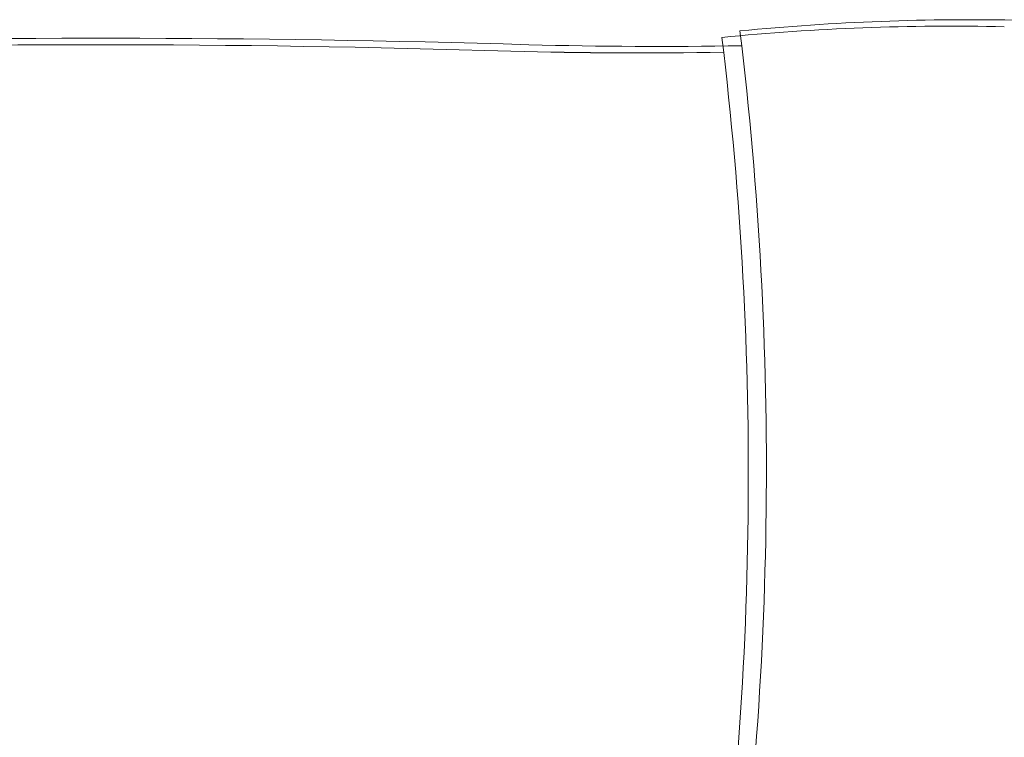
# Model space of a CAD drawing. Units: inches. Extents: x 1901 to 2863, y 888 to 2433.
# Tile 45 of 91: x 2686 to 2725, y 1595 to 1624. Entities that reach past the tile are written whole.
import ezdxf

# ---------------------------------------------------------------- set-up
doc = ezdxf.new("R2010")
doc.units = ezdxf.units.IN
doc.layers.add('A-FURN', color=8, linetype='Continuous', lineweight=18)

# ---------------------------------------------------------------- blocks, each defined once
blk = doc.blocks.new('BED-DOUBLE')
for centre, radius, start, end in [((176.248, 20.155), 144.857, 171.78449, 186.90062), ((176.248, 20.155), 144.857, 171.78449, 186.90062), ((175.53, 19.899), 144.857, 171.78449, 186.90062), ((175.53, 19.899), 144.857, 171.78449, 186.90062), ((35.744, -187.624), 190.991, 88.4762, 91.00819), ((35.744, -187.625), 190.991, 88.4762, 91.00819), ((57.571, 544.554), 541.514, 268.22771, 271.71854), ((57.571, 544.554), 541.514, 268.22771, 271.71854), ((23.307, 95.835), 93.531, 268.72178, 275.60397), ((23.307, 95.835), 93.531, 268.72178, 275.60397), ((35.026, -187.881), 190.991, 88.4762, 91.00819), ((35.026, -187.881), 190.991, 88.4762, 91.00819), ((56.853, 544.298), 541.514, 268.22771, 271.71854), ((56.853, 544.297), 541.514, 268.22771, 271.71854), ((22.589, 95.579), 93.531, 268.72178, 275.60397), ((22.589, 95.579), 93.531, 268.72178, 275.60397)]:
    blk.add_arc(centre, radius, start, end)

msp = doc.modelspace()

# ---------------------------------------------------------------- block references
at = {"layer": 'A-FURN', "rotation": 180}
msp.add_blockref('BED-DOUBLE', (2745.89, 1626.019), dxfattribs=at)

doc.saveas('drawing.dxf')
